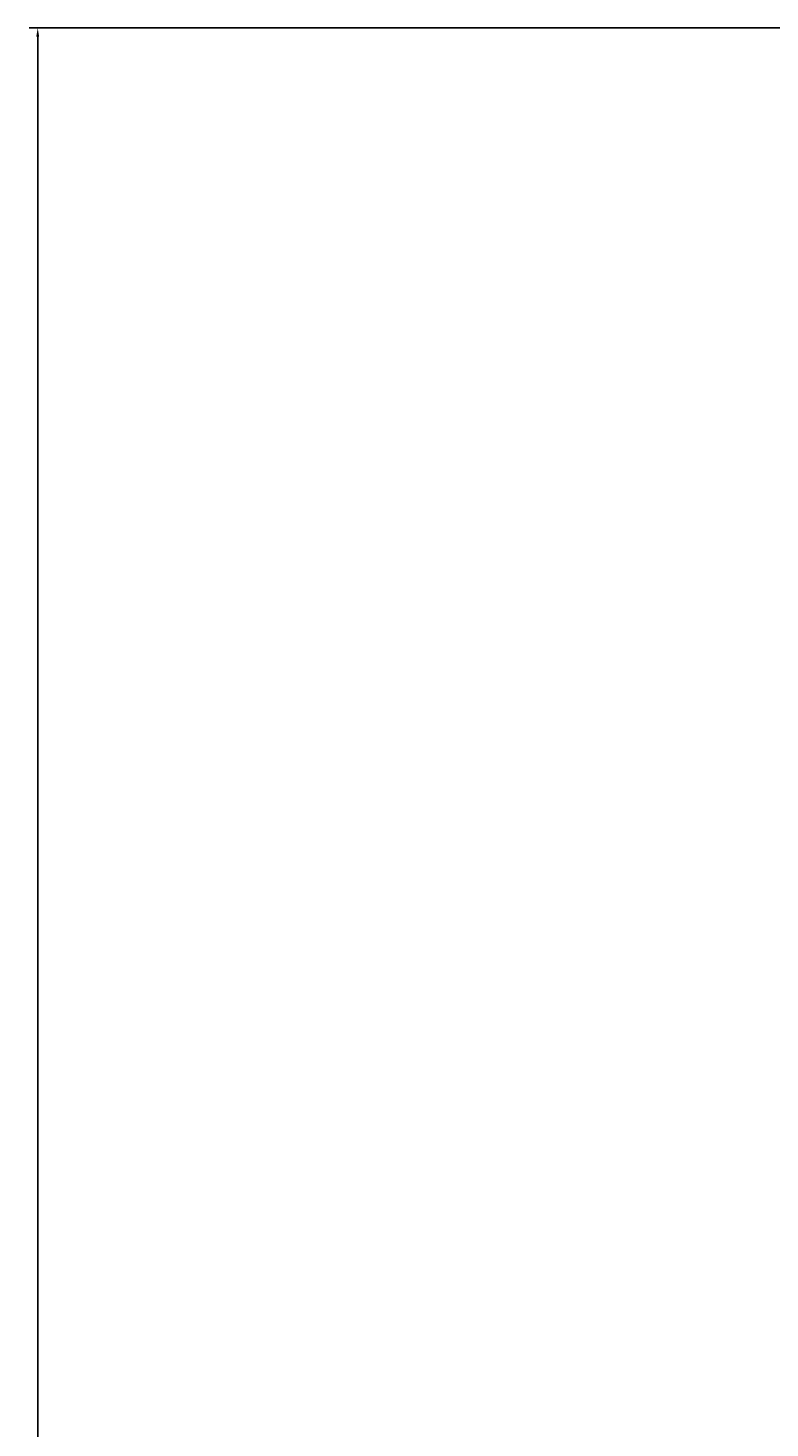
# Model space of a CAD drawing. Units: feet. Extents: x 2695 to 2912, y 795 to 1139.
# Tile 48 of 83: x 2695 to 2710, y 1093 to 1123. Entities that reach past the tile are written whole.
import ezdxf

# ---------------------------------------------------------------- set-up
doc = ezdxf.new("R2010")
doc.units = ezdxf.units.FT
doc.layers.add('A-ANNO-DIMS', color=2, linetype='Continuous', lineweight=18)
doc.styles.get("Standard").update_dxf_attribs({"font": 'arial.ttf'})
doc.dimstyles.get("Standard").update_dxf_attribs({"dimtxt": 0.18, "dimasz": 0.18, "dimexe": 0.18, "dimexo": 0.0625, "dimgap": 0.09, "dimtad": 0, "dimtih": 1, "dimtoh": 1, "dimdec": 1, "dimzin": 0, "dimdsep": 46, "dimlunit": 3, "dimtxsty": 'Standard', "dimcen": 0.09, "dimadec": 0, "dimazin": 0, "dimtfac": 1, "dimtdec": 1, "dimtofl": 0, "dimtmove": 0, "dimatfit": 3, "dimfxl": 1, "dimtolj": 1, "dimtzin": 0, "dimarcsym": 0})

# ---------------------------------------------------------------- blocks, each defined once
blk = doc.blocks.new('*D12')
at = {"layer": 'A-ANNO-DIMS', "color": 0, "lineweight": -2, "transparency": 16777216}
for p, q in [((2710.574, 1122.931), (2694.681, 1122.931)), ((2694.861, 1122.751), (2694.861, 967.113)), ((2694.861, 811.111), (2694.861, 966.749)), ((2710.574, 810.931), (2694.681, 810.931))]:
    blk.add_line(p, q, dxfattribs=at)
at = {"layer": 'A-ANNO-DIMS', "color": 0, "transparency": 16777216}
for points in [[(2694.831, 1122.751), (2694.891, 1122.751), (2694.861, 1122.931)], [(2694.831, 811.111), (2694.891, 811.111), (2694.861, 810.931)]]:
    blk.add_solid(points, dxfattribs=at)
at = {"layer": 'Defpoints', "color": 0, "transparency": 16777216}
for p in [(2694.861, 1122.931), (2710.636, 1122.931), (2710.636, 810.931)]:
    blk.add_point(p, dxfattribs=at)
at = {"layer": 'A-ANNO-DIMS', "color": 0, "transparency": 16777216, "insert": (2694.861, 966.931), "char_height": 0.18, "attachment_point": 5}
blk.add_mtext('\\A1;312', dxfattribs=at)

msp = doc.modelspace()

# ---------------------------------------------------------------- dimensions: what is measured, and where the dimension line sits
at = {"layer": 'A-ANNO-DIMS'}
dim = msp.add_linear_dim(base=(2694.8611, 1122.9306), p1=(2710.6361, 810.9306), p2=(2710.6361, 1122.9306), angle=90, dimstyle='Standard', override={"dimdec": 0, "dimlfac": 1, "dimrnd": 0, "dimzin": 0, "dimdsep": 46, "dimlunit": 2}, dxfattribs=at)
dim.commit()
dim.dimension.update_dxf_attribs({"geometry": '*D12', "text_midpoint": (2694.8611, 966.9306)})

doc.saveas('drawing.dxf')
